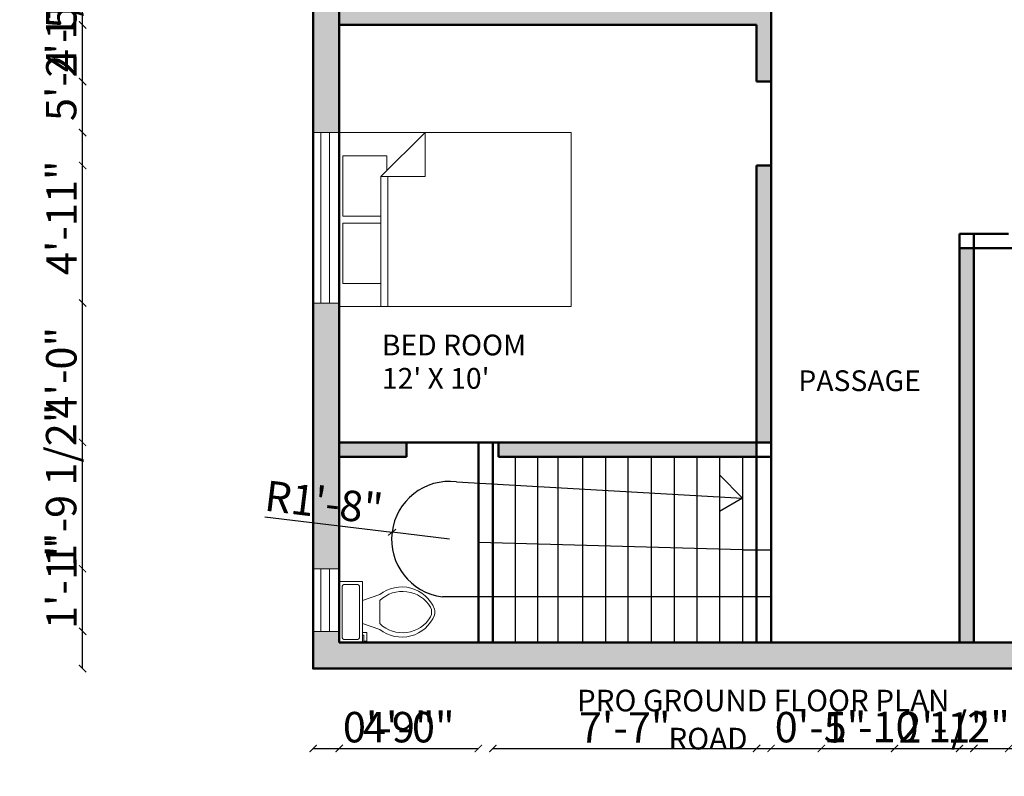
# Model space of a CAD drawing. Units: inches. Extents: x 1699 to 2290, y 1404 to 1978.
# Tile 1 of 4: x 1747 to 2086, y 1404 to 1665. Entities that reach past the tile are written whole.
import ezdxf

# ---------------------------------------------------------------- set-up
doc = ezdxf.new("R2010")
doc.units = ezdxf.units.IN
for name, color, linetype, lineweight in [('A-ANNO-DIMS', 2, 'Continuous', 18), ('A-ANNO-TEXT', 7, 'Continuous', 25), ('A-AREA-IDEN', 7, 'Continuous', 25), ('A-FLOR-FIXT', 9, 'Continuous', 18), ('A-FLOR-STRS', 7, 'Continuous', 25), ('A-FURN', 8, 'Continuous', 18), ('A-WALL', 7, 'Continuous', 50), ('A-WALL-PATT', 17, 'Continuous', 13), ('window', 3, 'Continuous', 18)]:
    doc.layers.add(name, color=color, linetype=linetype, lineweight=lineweight)
doc.styles.get("Standard").update_dxf_attribs({"font": 'arial.ttf'})
doc.dimstyles.new('ISO-25', dxfattribs={"dimtxt": 10.5, "dimasz": 2.5, "dimexe": 1.25, "dimexo": 0.625, "dimtad": 1, "dimdec": 0, "dimlunit": 4, "dimtxsty": 'Standard', "dimblk": 'ARCHTICK', "dimcen": 2.5, "dimse1": 1, "dimse2": 1, "dimclrd": 4, "dimclrt": 2, "dimadec": 0, "dimazin": 0, "dimtfac": 1, "dimtdec": 0, "dimtmove": 0, "dimatfit": 3, "dimfxl": 1, "dimarcsym": 0})

# ---------------------------------------------------------------- blocks, each defined once
blk = doc.blocks.new('Bed - Queen')
for p, q in [((0, -80.00003), (0, 0)), ((0, 0), (59.99999, 0)), ((59.99999, 0), (59.99999, -80.00003)), ((7.99999, -1.2), (28.79998, -1.2)), ((7.99999, -14.4), (7.99999, -1.2)), ((28.79998, -1.2), (28.79998, -14.4)), ((31.19999, -1.2), (51.99999, -1.2)), ((31.19999, -14.4), (31.19999, -1.2)), ((51.99999, -1.2), (51.99999, -16.4)), ((0, -14.4), (44.8, -14.4)), ((44.8, -16.8), (0, -16.8)), ((59.99999, -29.6), (44.8, -14.4)), ((44.8, -14.4), (44.8, -29.6)), ((51.99999, -16.4), (46.79936, -16.4)), ((44.8, -29.6), (59.99999, -29.6)), ((59.99999, -80.00003), (0, -80.00003))]:
    blk.add_line(p, q)
blk = doc.blocks.new('*U3')
for p, q in [((9.5, -6), (9.5, -2)), ((-10, -8.5), (-8, -8.5)), ((-10, -9.5), (-10, -8.5)), ((-7, -9.5), (-10, -9.5)), ((-8, -8.5), (-8, -8)), ((-7, -8), (-7, -9.5)), ((-4, -8), (-6, -14)), ((4, -8), (6, -14)), ((4, -14), (-4, -14))]:
    blk.add_line(p, q)
blk.add_lwpolyline([(10.5, -8), (10.5, 0), (-10.5, 0), (-10.5, -8)], close=True)
for points in [[(-9.5, -2), (-9.5, -6)], [(8.5, -1), (-8.5, -1)], [(-8.5, -7), (8.5, -7)]]:
    blk.add_lwpolyline(points)
for centre, radius, start, end in [((-8.62, -1.88), 0.884, 81.8699, 188.1301), ((8.62, -1.88), 0.884, 351.8699, 98.1301), ((-8.62, -6.12), 0.884, 171.8699, 278.1301), ((8.62, -6.12), 0.884, 261.8699, 8.1301), ((3.52, -21.58), 12.17, 141.4691, 247.9714), ((4.2, -21.82), 11.33, 136.3677, 238.9468), ((-3.52, -21.58), 12.17, 292.0284, 38.5307), ((-4.2, -21.82), 11.33, 301.053, 43.6321), ((0, -27.88), 4, 245.7318, 294.2682), ((0, -29), 4, 254.8605, 285.1395)]:
    blk.add_arc(centre, radius, start, end)
blk = doc.blocks.new('_ArchTick')
at = {"color": 0, "linetype": 'ByBlock', "const_width": 0.15}
blk.add_lwpolyline([(-0.5, -0.5), (0.5, 0.5)], dxfattribs=at)
blk = doc.blocks.new('*D24')
at = {"layer": 'A-ANNO-DIMS', "color": 4, "lineweight": -2, "transparency": 16777216}
for p, q in [((1847.82, 1414.03), (1856.82, 1414.03)), ((1856.82, 1414.03), (1888.48, 1414.03))]:
    blk.add_line(p, q, dxfattribs=at)
at = {"layer": 'Defpoints', "color": 0, "transparency": 16777216}
for p in [(1856.82, 1450.58), (1847.82, 1441.58), (1856.82, 1414.03)]:
    blk.add_point(p, dxfattribs=at)
at = {"layer": 'A-ANNO-DIMS', "color": 4, "lineweight": -2, "transparency": 16777216, "xscale": 2.5, "yscale": 2.5, "zscale": 2.5, "rotation": 180}
blk.add_blockref('_ArchTick', (1847.82, 1414.03), dxfattribs=at)
at = {"layer": 'A-ANNO-DIMS', "color": 4, "lineweight": -2, "transparency": 16777216, "xscale": 2.5, "yscale": 2.5, "zscale": 2.5}
blk.add_blockref('_ArchTick', (1856.82, 1414.03), dxfattribs=at)
at = {"layer": 'A-ANNO-DIMS', "color": 2, "transparency": 16777216, "insert": (1873.9, 1420.02), "char_height": 10.5, "attachment_point": 5}
blk.add_mtext('0\'-9"', dxfattribs=at)
blk = doc.blocks.new('*D25')
at = {"layer": 'A-ANNO-DIMS', "color": 4, "lineweight": -2, "transparency": 16777216}
blk.add_line((1856.82, 1414.03), (1904.82, 1414.03), dxfattribs=at)
at = {"layer": 'Defpoints', "color": 0, "transparency": 16777216}
for p in [(1856.82, 1450.58), (1904.82, 1450.58), (1904.82, 1414.03)]:
    blk.add_point(p, dxfattribs=at)
at = {"layer": 'A-ANNO-DIMS', "color": 4, "lineweight": -2, "transparency": 16777216, "xscale": 2.5, "yscale": 2.5, "zscale": 2.5, "rotation": 180}
blk.add_blockref('_ArchTick', (1856.82, 1414.03), dxfattribs=at)
at = {"layer": 'A-ANNO-DIMS', "color": 4, "lineweight": -2, "transparency": 16777216, "xscale": 2.5, "yscale": 2.5, "zscale": 2.5}
blk.add_blockref('_ArchTick', (1904.82, 1414.03), dxfattribs=at)
at = {"layer": 'A-ANNO-DIMS', "color": 2, "transparency": 16777216, "insert": (1880.82, 1420.02), "char_height": 10.5, "attachment_point": 5}
blk.add_mtext('4\'-0"', dxfattribs=at)
blk = doc.blocks.new('*D26')
at = {"layer": 'A-ANNO-DIMS', "color": 4, "lineweight": -2, "transparency": 16777216}
blk.add_line((1909.821631, 1414.034885), (2000.821631, 1414.034885), dxfattribs=at)
at = {"layer": 'Defpoints', "color": 0, "transparency": 16777216}
for p in [(1909.821631, 1450.584885), (2000.821631, 1450.584885), (2000.821631, 1414.034885)]:
    blk.add_point(p, dxfattribs=at)
at = {"layer": 'A-ANNO-DIMS', "color": 4, "lineweight": -2, "transparency": 16777216, "xscale": 2.5, "yscale": 2.5, "zscale": 2.5, "rotation": 180}
blk.add_blockref('_ArchTick', (1909.821631, 1414.034885), dxfattribs=at)
at = {"layer": 'A-ANNO-DIMS', "color": 4, "lineweight": -2, "transparency": 16777216, "xscale": 2.5, "yscale": 2.5, "zscale": 2.5}
blk.add_blockref('_ArchTick', (2000.821631, 1414.034885), dxfattribs=at)
at = {"layer": 'A-ANNO-DIMS', "color": 2, "transparency": 16777216, "insert": (1955.321631, 1419.909885), "char_height": 10.5, "attachment_point": 5}
blk.add_mtext('7\'-7"', dxfattribs=at)
blk = doc.blocks.new('*D27')
at = {"layer": 'A-ANNO-DIMS', "color": 4, "lineweight": -2, "transparency": 16777216}
blk.add_line((2005.82, 1949.13), (2070.82, 1949.13), dxfattribs=at)
at = {"layer": 'Defpoints', "color": 0, "transparency": 16777216}
for p in [(2070.82, 1949.13), (2005.82, 1450.58), (2070.82, 1450.58)]:
    blk.add_point(p, dxfattribs=at)
at = {"layer": 'A-ANNO-DIMS', "color": 4, "lineweight": -2, "transparency": 16777216, "xscale": 2.5, "yscale": 2.5, "zscale": 2.5, "rotation": 180}
blk.add_blockref('_ArchTick', (2005.82, 1949.13), dxfattribs=at)
at = {"layer": 'A-ANNO-DIMS', "color": 4, "lineweight": -2, "transparency": 16777216, "xscale": 2.5, "yscale": 2.5, "zscale": 2.5}
blk.add_blockref('_ArchTick', (2070.82, 1949.13), dxfattribs=at)
at = {"layer": 'A-ANNO-DIMS', "color": 2, "transparency": 16777216, "insert": (2038.32, 1955.1), "char_height": 10.5, "attachment_point": 5}
blk.add_mtext('5\'-5"', dxfattribs=at)
blk = doc.blocks.new('*D28')
at = {"layer": 'A-ANNO-DIMS', "color": 4, "lineweight": -2, "transparency": 16777216}
for p, q in [((1768.27, 1454.43), (1768.27, 1485.1)), ((1768.27, 1441.58), (1768.27, 1454.43))]:
    blk.add_line(p, q, dxfattribs=at)
at = {"layer": 'Defpoints', "color": 0, "transparency": 16777216}
for p in [(1768.27, 1454.43), (1847.82, 1454.43), (1847.82, 1441.58)]:
    blk.add_point(p, dxfattribs=at)
at = {"layer": 'A-ANNO-DIMS', "color": 4, "lineweight": -2, "transparency": 16777216, "xscale": 2.5, "yscale": 2.5, "zscale": 2.5}
for p, rotation in [((1768.27, 1454.43), 90), ((1768.27, 1441.58), 270)]:
    blk.add_blockref('_ArchTick', p, dxfattribs=dict(at, rotation=rotation))
at = {"layer": 'A-ANNO-DIMS', "color": 2, "transparency": 16777216, "insert": (1762.38, 1471.02), "char_height": 10.5, "attachment_point": 5, "rotation": 90}
blk.add_mtext('1\'-1"', dxfattribs=at)
blk = doc.blocks.new('*D29')
at = {"layer": 'A-ANNO-DIMS', "color": 4, "lineweight": -2, "transparency": 16777216}
for p, q in [((1768.27, 1476), (1768.27, 1531.14)), ((1768.27, 1454.43), (1768.27, 1476))]:
    blk.add_line(p, q, dxfattribs=at)
at = {"layer": 'Defpoints', "color": 0, "transparency": 16777216}
for p in [(1768.27, 1476), (1847.82, 1476), (1847.82, 1454.43)]:
    blk.add_point(p, dxfattribs=at)
at = {"layer": 'A-ANNO-DIMS', "color": 4, "lineweight": -2, "transparency": 16777216, "xscale": 2.5, "yscale": 2.5, "zscale": 2.5}
for p, rotation in [((1768.27, 1476), 90), ((1768.27, 1454.43), 270)]:
    blk.add_blockref('_ArchTick', p, dxfattribs=dict(at, rotation=rotation))
at = {"layer": 'A-ANNO-DIMS', "color": 2, "transparency": 16777216, "insert": (1762.22, 1504.82), "char_height": 10.5, "attachment_point": 5, "rotation": 90}
blk.add_mtext('1\'-9 1/2"', dxfattribs=at)
blk = doc.blocks.new('*D30')
at = {"layer": 'A-ANNO-DIMS', "color": 4, "lineweight": -2, "transparency": 16777216}
blk.add_line((1768.27, 1519.58), (1768.27, 1567.67), dxfattribs=at)
at = {"layer": 'Defpoints', "color": 0, "transparency": 16777216}
for p in [(1768.27, 1567.67), (1847.82, 1567.67), (1856.82, 1519.58)]:
    blk.add_point(p, dxfattribs=at)
at = {"layer": 'A-ANNO-DIMS', "color": 4, "lineweight": -2, "transparency": 16777216, "xscale": 2.5, "yscale": 2.5, "zscale": 2.5}
for p, rotation in [((1768.27, 1567.67), 90), ((1768.27, 1519.58), 270)]:
    blk.add_blockref('_ArchTick', p, dxfattribs=dict(at, rotation=rotation))
at = {"layer": 'A-ANNO-DIMS', "color": 2, "transparency": 16777216, "insert": (1762.29, 1543.63), "char_height": 10.5, "attachment_point": 5, "rotation": 90}
blk.add_mtext('4\'-0"', dxfattribs=at)
blk = doc.blocks.new('*D31')
at = {"layer": 'A-ANNO-DIMS', "color": 4, "lineweight": -2, "transparency": 16777216}
blk.add_line((1768.27, 1567.67), (1768.27, 1626.46), dxfattribs=at)
at = {"layer": 'Defpoints', "color": 0, "transparency": 16777216}
for p in [(1768.27, 1626.46), (1847.82, 1626.46), (1847.82, 1567.67)]:
    blk.add_point(p, dxfattribs=at)
at = {"layer": 'A-ANNO-DIMS', "color": 4, "lineweight": -2, "transparency": 16777216, "xscale": 2.5, "yscale": 2.5, "zscale": 2.5}
for p, rotation in [((1768.27, 1626.46), 90), ((1768.27, 1567.67), 270)]:
    blk.add_blockref('_ArchTick', p, dxfattribs=dict(at, rotation=rotation))
at = {"layer": 'A-ANNO-DIMS', "color": 2, "transparency": 16777216, "insert": (1762.38, 1597.07), "char_height": 10.5, "attachment_point": 5, "rotation": 90}
blk.add_mtext('4\'-11"', dxfattribs=at)
blk = doc.blocks.new('*D32')
at = {"layer": 'A-ANNO-DIMS', "color": 4, "lineweight": -2, "transparency": 16777216}
blk.add_line((1768.27, 1626.46), (1768.27, 1690.77), dxfattribs=at)
at = {"layer": 'Defpoints', "color": 0, "transparency": 16777216}
for p in [(1768.27, 1690.77), (1847.82, 1690.77), (1847.82, 1626.46)]:
    blk.add_point(p, dxfattribs=at)
at = {"layer": 'A-ANNO-DIMS', "color": 4, "lineweight": -2, "transparency": 16777216, "xscale": 2.5, "yscale": 2.5, "zscale": 2.5}
for p, rotation in [((1768.27, 1690.77), 90), ((1768.27, 1626.46), 270)]:
    blk.add_blockref('_ArchTick', p, dxfattribs=dict(at, rotation=rotation))
at = {"layer": 'A-ANNO-DIMS', "color": 2, "transparency": 16777216, "insert": (1762.22, 1658.62), "char_height": 10.5, "attachment_point": 5, "rotation": 90}
blk.add_mtext('5\'-4 1/2"', dxfattribs=at)
blk = doc.blocks.new('*D51')
at = {"layer": 'A-ANNO-DIMS', "color": 4, "lineweight": -2, "transparency": 16777216}
for p, q in [((1768.27, 1644.06), (1768.27, 1675.9)), ((1768.27, 1615.11), (1768.27, 1644.06))]:
    blk.add_line(p, q, dxfattribs=at)
at = {"layer": 'Defpoints', "color": 0, "transparency": 16777216}
for p in [(1768.27, 1644.06), (2000.82, 1644.06), (2000.82, 1615.11)]:
    blk.add_point(p, dxfattribs=at)
at = {"layer": 'A-ANNO-DIMS', "color": 4, "lineweight": -2, "transparency": 16777216, "xscale": 2.5, "yscale": 2.5, "zscale": 2.5}
for p, rotation in [((1768.27, 1644.06), 90), ((1768.27, 1615.11), 270)]:
    blk.add_blockref('_ArchTick', p, dxfattribs=dict(at, rotation=rotation))
at = {"layer": 'A-ANNO-DIMS', "color": 2, "transparency": 16777216, "insert": (1762.29, 1661.23), "char_height": 10.5, "attachment_point": 5, "rotation": 90}
blk.add_mtext('2\'-5"', dxfattribs=at)
blk = doc.blocks.new('*D52')
at = {"layer": 'A-ANNO-DIMS', "color": 4, "lineweight": -2, "transparency": 16777216}
for p, q in [((2023.18, 1414.03), (2048.43, 1414.03)), ((2048.43, 1414.03), (2080.27, 1414.03))]:
    blk.add_line(p, q, dxfattribs=at)
at = {"layer": 'Defpoints', "color": 0, "transparency": 16777216}
for p in [(2023.18, 1842.58), (2048.43, 1842.58), (2048.43, 1414.03)]:
    blk.add_point(p, dxfattribs=at)
at = {"layer": 'A-ANNO-DIMS', "color": 4, "lineweight": -2, "transparency": 16777216, "xscale": 2.5, "yscale": 2.5, "zscale": 2.5, "rotation": 180}
blk.add_blockref('_ArchTick', (2023.18, 1414.03), dxfattribs=at)
at = {"layer": 'A-ANNO-DIMS', "color": 4, "lineweight": -2, "transparency": 16777216, "xscale": 2.5, "yscale": 2.5, "zscale": 2.5}
blk.add_blockref('_ArchTick', (2048.43, 1414.03), dxfattribs=at)
at = {"layer": 'A-ANNO-DIMS', "color": 2, "transparency": 16777216, "insert": (2065.6, 1419.93), "char_height": 10.5, "attachment_point": 5}
blk.add_mtext('2\'-1"', dxfattribs=at)
blk = doc.blocks.new('*D55')
at = {"layer": 'A-ANNO-DIMS', "color": 4, "lineweight": -2, "transparency": 16777216}
for p, q in [((2000.82, 1414.03), (2005.82, 1414.03)), ((2005.82, 1414.03), (2037.48, 1414.03))]:
    blk.add_line(p, q, dxfattribs=at)
at = {"layer": 'Defpoints', "color": 0, "transparency": 16777216}
for p in [(2000.82, 1644.06), (2005.82, 1644.06), (2005.82, 1414.03)]:
    blk.add_point(p, dxfattribs=at)
at = {"layer": 'A-ANNO-DIMS', "color": 4, "lineweight": -2, "transparency": 16777216, "xscale": 2.5, "yscale": 2.5, "zscale": 2.5, "rotation": 180}
blk.add_blockref('_ArchTick', (2000.82, 1414.03), dxfattribs=at)
at = {"layer": 'A-ANNO-DIMS', "color": 4, "lineweight": -2, "transparency": 16777216, "xscale": 2.5, "yscale": 2.5, "zscale": 2.5}
blk.add_blockref('_ArchTick', (2005.82, 1414.03), dxfattribs=at)
at = {"layer": 'A-ANNO-DIMS', "color": 2, "transparency": 16777216, "insert": (2022.9, 1420.02), "char_height": 10.5, "attachment_point": 5}
blk.add_mtext('0\'-5"', dxfattribs=at)
blk = doc.blocks.new('*D56')
at = {"layer": 'A-ANNO-DIMS', "color": 4, "lineweight": -2, "transparency": 16777216}
for p, q in [((1880.06, 1949.13), (1911.72, 1949.13)), ((1911.72, 1949.13), (1968.03, 1949.13))]:
    blk.add_line(p, q, dxfattribs=at)
at = {"layer": 'Defpoints', "color": 0, "transparency": 16777216}
for p in [(1911.72, 1949.13), (1880.06, 1519.58), (1911.72, 1519.58)]:
    blk.add_point(p, dxfattribs=at)
at = {"layer": 'A-ANNO-DIMS', "color": 4, "lineweight": -2, "transparency": 16777216, "xscale": 2.5, "yscale": 2.5, "zscale": 2.5, "rotation": 180}
blk.add_blockref('_ArchTick', (1880.06, 1949.13), dxfattribs=at)
at = {"layer": 'A-ANNO-DIMS', "color": 4, "lineweight": -2, "transparency": 16777216, "xscale": 2.5, "yscale": 2.5, "zscale": 2.5}
blk.add_blockref('_ArchTick', (1911.72, 1949.13), dxfattribs=at)
at = {"layer": 'A-ANNO-DIMS', "color": 2, "transparency": 16777216, "insert": (1941.12, 1955.19), "char_height": 10.5, "attachment_point": 5}
blk.add_mtext('2\'-7 1/2"', dxfattribs=at)
blk = doc.blocks.new('*D57')
at = {"layer": 'A-ANNO-DIMS', "color": 4, "lineweight": -2, "transparency": 16777216}
blk.add_line((1856.82, 1949.13), (1889.82, 1949.13), dxfattribs=at)
at = {"layer": 'Defpoints', "color": 0, "transparency": 16777216}
for p in [(1889.82, 1949.13), (1856.82, 1471.58), (1889.82, 1461.08)]:
    blk.add_point(p, dxfattribs=at)
at = {"layer": 'A-ANNO-DIMS', "color": 4, "lineweight": -2, "transparency": 16777216, "xscale": 2.5, "yscale": 2.5, "zscale": 2.5, "rotation": 180}
blk.add_blockref('_ArchTick', (1856.82, 1949.13), dxfattribs=at)
at = {"layer": 'A-ANNO-DIMS', "color": 4, "lineweight": -2, "transparency": 16777216, "xscale": 2.5, "yscale": 2.5, "zscale": 2.5}
blk.add_blockref('_ArchTick', (1889.82, 1949.13), dxfattribs=at)
at = {"layer": 'A-ANNO-DIMS', "color": 2, "transparency": 16777216, "insert": (1873.32, 1955.12), "char_height": 10.5, "attachment_point": 5}
blk.add_mtext('2\'-9"', dxfattribs=at)
blk = doc.blocks.new('*D58')
at = {"layer": 'A-ANNO-DIMS', "color": 4, "lineweight": -2, "transparency": 16777216}
for p, q in [((2235.37, 1471.58), (2235.37, 1502.26)), ((2235.37, 1450.58), (2235.37, 1471.58))]:
    blk.add_line(p, q, dxfattribs=at)
at = {"layer": 'Defpoints', "color": 0, "transparency": 16777216}
for p in [(1864.82, 1471.58), (2235.37, 1471.58), (1864.82, 1450.58)]:
    blk.add_point(p, dxfattribs=at)
at = {"layer": 'A-ANNO-DIMS', "color": 4, "lineweight": -2, "transparency": 16777216, "xscale": 2.5, "yscale": 2.5, "zscale": 2.5}
for p, rotation in [((2235.37, 1471.58), 90), ((2235.37, 1450.58), 270)]:
    blk.add_blockref('_ArchTick', p, dxfattribs=dict(at, rotation=rotation))
at = {"layer": 'A-ANNO-DIMS', "color": 2, "transparency": 16777216, "insert": (2229.39, 1488.17), "char_height": 10.5, "attachment_point": 5, "rotation": 90}
blk.add_mtext('1\'-9"', dxfattribs=at)
blk = doc.blocks.new('*D59')
at = {"layer": 'A-ANNO-DIMS', "color": 4, "lineweight": -2, "transparency": 16777216}
for p, q in [((1917.51, 1949.13), (1925.23, 1949.13)), ((1925.23, 1949.13), (1981.36, 1949.13))]:
    blk.add_line(p, q, dxfattribs=at)
at = {"layer": 'Defpoints', "color": 0, "transparency": 16777216}
for p in [(1925.23, 1949.13), (1917.51, 1514.58), (1925.23, 1514.58)]:
    blk.add_point(p, dxfattribs=at)
at = {"layer": 'A-ANNO-DIMS', "color": 4, "lineweight": -2, "transparency": 16777216, "xscale": 2.5, "yscale": 2.5, "zscale": 2.5, "rotation": 180}
blk.add_blockref('_ArchTick', (1917.51, 1949.13), dxfattribs=at)
at = {"layer": 'A-ANNO-DIMS', "color": 4, "lineweight": -2, "transparency": 16777216, "xscale": 2.5, "yscale": 2.5, "zscale": 2.5}
blk.add_blockref('_ArchTick', (1925.23, 1949.13), dxfattribs=at)
at = {"layer": 'A-ANNO-DIMS', "color": 2, "transparency": 16777216, "insert": (1954.55, 1955.19), "char_height": 10.5, "attachment_point": 5}
blk.add_mtext('0\'-7 1/2"', dxfattribs=at)
blk = doc.blocks.new('*D60')
at = {"layer": 'A-ANNO-DIMS', "color": 4, "lineweight": -2, "transparency": 16777216}
blk.add_line((2235.37, 1441.58), (2235.37, 1519.58), dxfattribs=at)
at = {"layer": 'Defpoints', "color": 0, "transparency": 16777216}
for p in [(2005.82, 1519.58), (2235.37, 1519.58), (1847.82, 1441.58)]:
    blk.add_point(p, dxfattribs=at)
at = {"layer": 'A-ANNO-DIMS', "color": 4, "lineweight": -2, "transparency": 16777216, "xscale": 2.5, "yscale": 2.5, "zscale": 2.5}
for p, rotation in [((2235.37, 1519.58), 90), ((2235.37, 1441.58), 270)]:
    blk.add_blockref('_ArchTick', p, dxfattribs=dict(at, rotation=rotation))
at = {"layer": 'A-ANNO-DIMS', "color": 2, "transparency": 16777216, "insert": (2229.39, 1480.58), "char_height": 10.5, "attachment_point": 5, "rotation": 90}
blk.add_mtext('6\'-6"', dxfattribs=at)
blk = doc.blocks.new('*D61')
at = {"layer": 'A-ANNO-DIMS', "color": 4, "lineweight": -2, "transparency": 16777216}
for p, q in [((2000.82, 1414.03), (2023.18, 1414.03)), ((2023.18, 1414.03), (2086.48, 1414.03))]:
    blk.add_line(p, q, dxfattribs=at)
at = {"layer": 'Defpoints', "color": 0, "transparency": 16777216}
for p in [(2000.82, 1842.58), (2023.18, 1842.58), (2023.18, 1414.03)]:
    blk.add_point(p, dxfattribs=at)
at = {"layer": 'A-ANNO-DIMS', "color": 4, "lineweight": -2, "transparency": 16777216, "xscale": 2.5, "yscale": 2.5, "zscale": 2.5, "rotation": 180}
blk.add_blockref('_ArchTick', (2000.82, 1414.03), dxfattribs=at)
at = {"layer": 'A-ANNO-DIMS', "color": 4, "lineweight": -2, "transparency": 16777216, "xscale": 2.5, "yscale": 2.5, "zscale": 2.5}
blk.add_blockref('_ArchTick', (2023.18, 1414.03), dxfattribs=at)
at = {"layer": 'A-ANNO-DIMS', "color": 2, "transparency": 16777216, "insert": (2056.08, 1420.09), "char_height": 10.5, "attachment_point": 5}
blk.add_mtext('1\'-10 1/2"', dxfattribs=at)
blk = doc.blocks.new('*D62')
at = {"layer": 'A-ANNO-DIMS', "color": 4, "lineweight": -2, "transparency": 16777216}
for p, q in [((2070.82, 1414.03), (2087.8, 1414.03)), ((2087.8, 1414.03), (2118.47, 1414.03))]:
    blk.add_line(p, q, dxfattribs=at)
at = {"layer": 'Defpoints', "color": 0, "transparency": 16777216}
for p in [(2070.82, 1586.58), (2087.8, 1586.58), (2087.8, 1414.03)]:
    blk.add_point(p, dxfattribs=at)
at = {"layer": 'A-ANNO-DIMS', "color": 4, "lineweight": -2, "transparency": 16777216, "xscale": 2.5, "yscale": 2.5, "zscale": 2.5, "rotation": 180}
blk.add_blockref('_ArchTick', (2070.82, 1414.03), dxfattribs=at)
at = {"layer": 'A-ANNO-DIMS', "color": 4, "lineweight": -2, "transparency": 16777216, "xscale": 2.5, "yscale": 2.5, "zscale": 2.5}
blk.add_blockref('_ArchTick', (2087.8, 1414.03), dxfattribs=at)
at = {"layer": 'A-ANNO-DIMS', "color": 2, "transparency": 16777216, "insert": (2104.39, 1420.02), "char_height": 10.5, "attachment_point": 5}
blk.add_mtext('1\'-5"', dxfattribs=at)
blk = doc.blocks.new('*D63')
at = {"layer": 'A-ANNO-DIMS', "color": 4, "lineweight": -2, "transparency": 16777216}
for p, q in [((1768.27, 1663.58), (1768.27, 1718.72)), ((1768.27, 1644.06), (1768.27, 1663.58))]:
    blk.add_line(p, q, dxfattribs=at)
at = {"layer": 'Defpoints', "color": 0, "transparency": 16777216}
for p in [(1768.27, 1663.58), (2000.82, 1663.58), (2000.82, 1644.06)]:
    blk.add_point(p, dxfattribs=at)
at = {"layer": 'A-ANNO-DIMS', "color": 4, "lineweight": -2, "transparency": 16777216, "xscale": 2.5, "yscale": 2.5, "zscale": 2.5}
for p, rotation in [((1768.27, 1663.58), 90), ((1768.27, 1644.06), 270)]:
    blk.add_blockref('_ArchTick', p, dxfattribs=dict(at, rotation=rotation))
at = {"layer": 'A-ANNO-DIMS', "color": 2, "transparency": 16777216, "insert": (1762.22, 1692.4), "char_height": 10.5, "attachment_point": 5, "rotation": 90}
blk.add_mtext('1\'-7 1/2"', dxfattribs=at)
blk = doc.blocks.new('*D65')
at = {"layer": 'A-ANNO-DIMS', "color": 4, "lineweight": -2, "transparency": 16777216}
for p, q in [((1856.82, 1949.13), (1880.06, 1949.13)), ((1880.06, 1949.13), (1918.89, 1949.13))]:
    blk.add_line(p, q, dxfattribs=at)
at = {"layer": 'Defpoints', "color": 0, "transparency": 16777216}
for p in [(1880.06, 1949.13), (1856.82, 1519.58), (1880.06, 1519.58)]:
    blk.add_point(p, dxfattribs=at)
at = {"layer": 'A-ANNO-DIMS', "color": 4, "lineweight": -2, "transparency": 16777216, "xscale": 2.5, "yscale": 2.5, "zscale": 2.5, "rotation": 180}
blk.add_blockref('_ArchTick', (1856.82, 1949.13), dxfattribs=at)
at = {"layer": 'A-ANNO-DIMS', "color": 4, "lineweight": -2, "transparency": 16777216, "xscale": 2.5, "yscale": 2.5, "zscale": 2.5}
blk.add_blockref('_ArchTick', (1880.06, 1949.13), dxfattribs=at)
at = {"layer": 'A-ANNO-DIMS', "color": 2, "transparency": 16777216, "insert": (1900.72, 1955.03), "char_height": 10.5, "attachment_point": 5}
blk.add_mtext('1\'-11"', dxfattribs=at)
blk = doc.blocks.new('*D67')
at = {"layer": 'A-ANNO-DIMS', "color": 4, "lineweight": -2, "transparency": 16777216}
for p, q in [((2075.82, 1414.03), (2103.12, 1414.03)), ((2103.12, 1414.03), (2159.43, 1414.03))]:
    blk.add_line(p, q, dxfattribs=at)
at = {"layer": 'Defpoints', "color": 0, "transparency": 16777216}
for p in [(2075.82, 1912.58), (2103.12, 1883.78), (2103.12, 1414.03)]:
    blk.add_point(p, dxfattribs=at)
at = {"layer": 'A-ANNO-DIMS', "color": 4, "lineweight": -2, "transparency": 16777216, "xscale": 2.5, "yscale": 2.5, "zscale": 2.5, "rotation": 180}
blk.add_blockref('_ArchTick', (2075.82, 1414.03), dxfattribs=at)
at = {"layer": 'A-ANNO-DIMS', "color": 4, "lineweight": -2, "transparency": 16777216, "xscale": 2.5, "yscale": 2.5, "zscale": 2.5}
blk.add_blockref('_ArchTick', (2103.12, 1414.03), dxfattribs=at)
at = {"layer": 'A-ANNO-DIMS', "color": 2, "transparency": 16777216, "insert": (2132.53, 1420.09), "char_height": 10.5, "attachment_point": 5}
blk.add_mtext('2\'-3 1/2"', dxfattribs=at)
blk = doc.blocks.new('*D70')
at = {"layer": 'A-ANNO-DIMS', "color": 4, "lineweight": -2, "transparency": 16777216}
for p in [(1831.16, 1493.95), (1894.84, 1486.18)]:
    blk.add_line(p, (1875.04, 1488.6), dxfattribs=at)
at = {"layer": 'Defpoints', "color": 0, "transparency": 16777216}
for p in [(1875.04, 1488.6), (1894.84, 1486.18)]:
    blk.add_point(p, dxfattribs=at)
at = {"layer": 'A-ANNO-DIMS', "color": 4, "lineweight": -2, "transparency": 16777216, "xscale": 2.5, "yscale": 2.5, "zscale": 2.5, "rotation": 353.0375972592239}
blk.add_blockref('_ArchTick', (1875.04, 1488.6), dxfattribs=at)
at = {"layer": 'A-ANNO-DIMS', "color": 2, "transparency": 16777216, "insert": (1851.35, 1497.52), "char_height": 10.5, "attachment_point": 5, "rotation": 353.0376}
blk.add_mtext('R1\'-8"', dxfattribs=at)

msp = doc.modelspace()

# ---------------------------------------------------------------- hatches: boundary and pattern name
at = {"layer": 'A-WALL-PATT'}
h = msp.add_hatch(color=256, dxfattribs=at)
h.dxf.hatch_style = 1
h.paths.add_polyline_path([(1893.7, 1921.58), (1847.82, 1921.58), (1847.82, 1852.66), (1856.82, 1852.66), (1856.82, 1912.58), (1893.7, 1912.58)])
h.paths.add_polyline_path([(2097.62, 1921.58), (1942.38, 1921.58), (1942.38, 1912.58), (2097.62, 1912.58)])
h.paths.add_polyline_path([(2207.82, 1921.58), (2149.1, 1921.58), (2149.1, 1912.58), (2153.96, 1912.58), (2198.82, 1912.58), (2198.82, 1877.29), (2207.82, 1877.29)])
h.paths.add_polyline_path([(2207.82, 1827.84), (2198.82, 1827.84), (2198.82, 1815.84), (2198.82, 1807.65), (2198.82, 1726.54), (2207.82, 1726.54)])
h.paths.add_polyline_path([(2207.82, 1677.38), (2198.82, 1677.38), (2198.82, 1660.38), (2198.82, 1547.09), (2207.82, 1547.09)])
h.paths.add_polyline_path([(2207.82, 1478.94), (2198.82, 1478.94), (2198.82, 1450.58), (1856.82, 1450.58), (1856.82, 1454.43), (1847.82, 1454.43), (1847.82, 1441.58), (2207.82, 1441.58)])
h.paths.add_polyline_path([(1856.82, 1567.67), (1847.82, 1567.67), (1847.82, 1476), (1856.82, 1476)])
h.paths.add_polyline_path([(1856.82, 1690.28), (1855.82, 1690.28), (1855.82, 1690.33), (1847.82, 1690.77), (1847.82, 1626.46), (1856.82, 1626.46)])
h.paths.add_polyline_path([(1856.82, 1802.75), (1847.82, 1802.75), (1847.82, 1720.13), (1856.82, 1720.13)])
h.paths.add_polyline_path([(2000.82, 1740.58), (1856.82, 1740.58), (1856.82, 1735.58), (2000.82, 1735.58)])
h.paths.add_polyline_path([(2005.82, 1668.58), (2000.82, 1668.58), (1856.82, 1668.58), (1856.82, 1663.58), (2000.82, 1663.58), (2000.82, 1644.06), (2005.82, 1644.06)])
h.paths.add_polyline_path([(2005.82, 1746.92), (2000.82, 1746.92), (2000.82, 1694.4), (2005.82, 1694.4)])
h.paths.add_polyline_path([(1957.82, 1735.58), (1952.82, 1735.58), (1952.82, 1694.4), (1957.82, 1694.4)])
h.paths.add_polyline_path([(2005.82, 1842.58), (2000.82, 1842.58), (2000.82, 1776.01), (2005.82, 1776.01)])
h.paths.add_polyline_path([(2000.82, 1519.58), (1911.72, 1519.58), (1911.72, 1514.58), (2000.82, 1514.58)])
h.paths.add_polyline_path([(1880.06, 1519.58), (1856.82, 1519.58), (1856.82, 1514.58), (1880.06, 1514.58)])
h.paths.add_polyline_path([(2005.82, 1615.11), (2000.82, 1615.11), (2000.82, 1519.58), (2005.82, 1519.58)])
h.paths.add_polyline_path([(2075.82, 1586.58), (2070.82, 1586.58), (2070.82, 1450.58), (2075.82, 1450.58)])
h.paths.add_polyline_path([(2198.82, 1591.58), (2112.54, 1591.58), (2112.54, 1586.58), (2198.82, 1586.58)])
h.paths.add_polyline_path([(2075.82, 1912.58), (2070.82, 1912.58), (2070.82, 1847.58), (2075.82, 1847.58)])
h.paths.add_polyline_path([(2198.82, 1785.58), (2075.82, 1785.58), (2075.82, 1780.58), (2198.82, 1780.58)])
h.paths.add_polyline_path([(2075.82, 1842.58), (2070.82, 1842.58), (2070.82, 1825.42), (2075.82, 1825.42)])
h.paths.add_polyline_path([(2075.82, 1847.58), (2070.82, 1847.58), (2070.82, 1842.58), (2075.82, 1842.58)])
h.paths.add_polyline_path([(2070.82, 1847.58), (2048.43, 1847.58), (2048.43, 1842.58), (2070.82, 1842.58)])
h.paths.add_polyline_path([(2023.18, 1847.58), (2005.82, 1847.58), (2005.82, 1842.58), (2023.18, 1842.58)])
h.paths.add_polyline_path([(2005.82, 1912.58), (2000.82, 1912.58), (2000.82, 1847.58), (2005.82, 1847.58)])
h.paths.add_polyline_path([(2005.82, 1847.58), (2000.82, 1847.58), (2000.82, 1842.58), (2005.82, 1842.58)])
h.paths.add_polyline_path([(2075.82, 1793.79), (2070.82, 1793.79), (2070.82, 1785.58), (2075.82, 1785.58)])
h.paths.add_polyline_path([(2075.82, 1785.58), (2070.82, 1785.58), (2070.82, 1780.58), (2075.82, 1780.58)])
h.paths.add_polyline_path([(2088.5, 1836.17), (2134.05, 1836.17), (2134.05, 1847.15), (2088.5, 1847.15)], flags=9)
h.paths.add_polyline_path([(2088.47, 1847.66), (2136.12, 1847.66), (2136.12, 1858.78), (2088.47, 1858.78)], flags=9)
h.paths.add_polyline_path([(2012.58, 1874.96), (2055.33, 1874.96), (2055.33, 1885.9), (2012.58, 1885.9)], flags=9)
h.paths.add_polyline_path([(2012.55, 1886.44), (2050.21, 1886.44), (2050.21, 1897.57), (2012.55, 1897.57)], flags=9)
h.paths.add_polyline_path([(1873.22, 1882.94), (1924.28, 1882.94), (1924.28, 1893.74), (1873.22, 1893.74)], flags=9)
h.paths.add_polyline_path([(1873.17, 1894.28), (1931.39, 1894.28), (1931.39, 1905.41), (1873.17, 1905.41)], flags=9)

# ---------------------------------------------------------------- linework, layer by layer
at = {"layer": 'A-FLOR-STRS'}
for p, q in [((1917.51, 1514.58), (1917.51, 1450.58)), ((1925.23, 1514.58), (1925.23, 1450.58)), ((1932.21, 1514.58), (1932.21, 1450.58)), ((1940.79, 1514.58), (1940.79, 1450.58)), ((1948.73, 1514.58), (1948.73, 1450.58)), ((1956.39, 1514.58), (1956.39, 1450.58)), ((1964.47, 1514.58), (1964.47, 1450.58)), ((1972.4, 1514.58), (1972.4, 1450.58)), ((1980.17, 1514.58), (1980.17, 1450.58)), ((1988.02, 1514.58), (1988.02, 1450.58)), ((1996.02, 1514.58), (1996.02, 1450.58)), ((1897.26, 1505.98), (1996.02, 1500.39)), ((1996.02, 1500.39), (1988.02, 1508.45)), ((1988.02, 1508.45), (1996.02, 1500.39)), ((1996.02, 1500.39), (1988.02, 1495.76)), ((1996.02, 1482.58), (1904.82, 1485.08)), ((1996.02, 1482.58), (2005.82, 1482.58)), ((2005.82, 1466.38), (1892.43, 1466.38))]:
    msp.add_line(p, q, dxfattribs=at)
msp.add_arc((1894.84, 1486.18), 19.95, 83.037, 263.037, dxfattribs=at)
at = {"layer": 'A-WALL'}
for p, q in [((1856.82, 1450.58), (1856.82, 1912.58)), ((2005.82, 1450.58), (2005.82, 1912.58)), ((1856.82, 1663.58), (2000.82, 1663.58)), ((2000.82, 1644.06), (2000.82, 1663.58)), ((2005.82, 1644.06), (2000.82, 1644.06)), ((2000.82, 1450.58), (2000.82, 1615.11)), ((2005.82, 1615.11), (2000.82, 1615.11)), ((2070.82, 1450.58), (2070.82, 1591.58)), ((2070.82, 1591.58), (2087.8, 1591.58)), ((2075.82, 1450.58), (2075.82, 1591.58)), ((2070.82, 1586.58), (2198.82, 1586.58)), ((1856.82, 1519.58), (2005.82, 1519.58)), ((1880.06, 1514.58), (1880.06, 1519.58)), ((1904.82, 1450.58), (1904.82, 1519.58)), ((1909.82, 1450.58), (1909.82, 1519.58)), ((1911.72, 1514.58), (1911.72, 1519.58)), ((1856.82, 1514.58), (1880.06, 1514.58)), ((1911.72, 1514.58), (2005.82, 1514.58)), ((2198.82, 1450.58), (1856.82, 1450.58))]:
    msp.add_line(p, q, dxfattribs=at)
msp.add_lwpolyline([(1847.82, 1921.58), (2207.82, 1921.58), (2207.82, 1441.58), (1847.82, 1441.58)], close=True, dxfattribs=at)
at = {"layer": 'window'}
for p, q in [((1856.82, 1626.46), (1847.82, 1626.46)), ((1847.82, 1626.46), (1847.82, 1567.67)), ((1850.5, 1626.46), (1850.5, 1567.67)), ((1853.48, 1626.46), (1853.48, 1567.67)), ((1856.82, 1567.67), (1856.82, 1626.46)), ((1847.82, 1567.67), (1856.82, 1567.67)), ((1856.82, 1476), (1847.82, 1476)), ((1847.82, 1476), (1847.82, 1454.43)), ((1850.45, 1476), (1850.45, 1454.43)), ((1853.5, 1476), (1853.5, 1454.43)), ((1856.82, 1454.43), (1856.82, 1476)), ((1847.82, 1454.43), (1856.82, 1454.43))]:
    msp.add_line(p, q, dxfattribs=at)

# ---------------------------------------------------------------- block references
at = {"layer": 'A-FLOR-FIXT', "rotation": 90}
msp.add_blockref('*U3', (1856.82, 1461.08), dxfattribs=at)
at = {"layer": 'A-FURN', "rotation": 90}
msp.add_blockref('Bed - Queen', (1856.82, 1566.46), dxfattribs=at)

# ---------------------------------------------------------------- texts
at = {"layer": 'A-ANNO-TEXT'}
for s, p in [('PRO GROUND FLOOR PLAN', (1938.86, 1426.82)), ('ROAD', (1970.43, 1413.68))]:
    msp.add_text(s, height=7.476, dxfattribs=at).set_placement(p)
at = {"layer": 'A-AREA-IDEN'}
for s, p in [('BED ROOM', (1871.54, 1549.61)), ("12' X 10'", (1871.54, 1538.1)), ('PASSAGE', (2015.24, 1537.29))]:
    msp.add_text(s, height=7.167, dxfattribs=at).set_placement(p)

# ---------------------------------------------------------------- dimensions: what is measured, and where the dimension line sits
at = {"layer": 'A-ANNO-DIMS'}
for base, p1, p2, picture, middle in [((1911.72, 1949.13), (1880.06, 1519.58), (1911.72, 1519.58), '*D56', (1941.12, 1955.19)), ((1925.23, 1949.13), (1917.51, 1514.58), (1925.23, 1514.58), '*D59', (1954.55, 1955.19)), ((1889.82, 1949.13), (1856.82, 1471.58), (1889.82, 1461.08), '*D57', (1873.32, 1955.12)), ((1880.06, 1949.13), (1856.82, 1519.58), (1880.06, 1519.58), '*D65', (1900.72, 1955.03)), ((2070.82, 1949.13), (2005.82, 1450.58), (2070.82, 1450.58), '*D27', (2038.32, 1955.1)), ((2103.12, 1414.03), (2075.82, 1912.58), (2103.12, 1883.78), '*D67', (2132.53, 1420.09)), ((2023.18, 1414.03), (2000.82, 1842.58), (2023.18, 1842.58), '*D61', (2056.08, 1420.09)), ((2048.4251, 1414.0349), (2023.1812, 1842.5849), (2048.4251, 1842.5849), '*D52', (2065.5955, 1419.9314)), ((2005.82, 1414.03), (2000.82, 1644.06), (2005.82, 1644.06), '*D55', (2022.9, 1420.02)), ((2087.8, 1414.03), (2070.82, 1586.58), (2087.8, 1586.58), '*D62', (2104.39, 1420.02)), ((1856.82, 1414.03), (1847.82, 1441.58), (1856.82, 1450.58), '*D24', (1873.9, 1420.02)), ((1904.82, 1414.03), (1856.82, 1450.58), (1904.82, 1450.58), '*D25', (1880.82, 1420.02)), ((2000.82, 1414.03), (1909.82, 1450.58), (2000.82, 1450.58), '*D26', (1955.32, 1419.91))]:
    dim = msp.add_linear_dim(base=base, p1=p1, p2=p2, dimstyle='ISO-25', override={"dimdec": 1, "dimlfac": 1, "dimrnd": 0, "dimzin": 1, "dimdsep": 46, "dimlunit": 4, "dimfrac": 2}, dxfattribs=at)
    dim.commit()
    dim.dimension.update_dxf_attribs({"geometry": picture, "text_midpoint": middle})
for base, p1, p2, picture, middle in [((1768.27, 1663.58), (2000.82, 1644.06), (2000.82, 1663.58), '*D63', (1762.22, 1692.4)), ((1768.27, 1690.77), (1847.82, 1626.46), (1847.82, 1690.77), '*D32', (1762.22, 1658.62)), ((1768.2716, 1644.0554), (2000.8216, 1615.11), (2000.8216, 1644.0554), '*D51', (1762.2856, 1661.2258)), ((1768.27, 1626.46), (1847.82, 1567.67), (1847.82, 1626.46), '*D31', (1762.38, 1597.07)), ((1768.27, 1567.67), (1856.82, 1519.58), (1847.82, 1567.67), '*D30', (1762.29, 1543.63)), ((1768.27, 1476), (1847.82, 1454.43), (1847.82, 1476), '*D29', (1762.22, 1504.82)), ((2235.37, 1519.58), (1847.82, 1441.58), (2005.82, 1519.58), '*D60', (2229.39, 1480.58)), ((2235.37, 1471.58), (1864.82, 1450.58), (1864.82, 1471.58), '*D58', (2229.39, 1488.17)), ((1768.2716, 1454.4303), (1847.8216, 1441.5849), (1847.8216, 1454.4303), '*D28', (1762.3751, 1471.017))]:
    dim = msp.add_linear_dim(base=base, p1=p1, p2=p2, angle=90, dimstyle='ISO-25', override={"dimdec": 1, "dimlfac": 1, "dimrnd": 0, "dimzin": 1, "dimdsep": 46, "dimlunit": 4, "dimfrac": 2}, dxfattribs=at)
    dim.commit()
    dim.dimension.update_dxf_attribs({"geometry": picture, "text_midpoint": middle})
dim = msp.add_radius_dim(center=(1894.84, 1486.18), mpoint=(1875.04, 1488.6), dimstyle='ISO-25', override={"dimdec": 1, "dimlfac": 1, "dimrnd": 0, "dimzin": 1, "dimdsep": 46, "dimlunit": 4, "dimfrac": 2}, dxfattribs=at)
dim.commit()
dim.dimension.update_dxf_attribs({"geometry": '*D70', "text_midpoint": (1851.35, 1497.52)})

doc.saveas('drawing.dxf')
